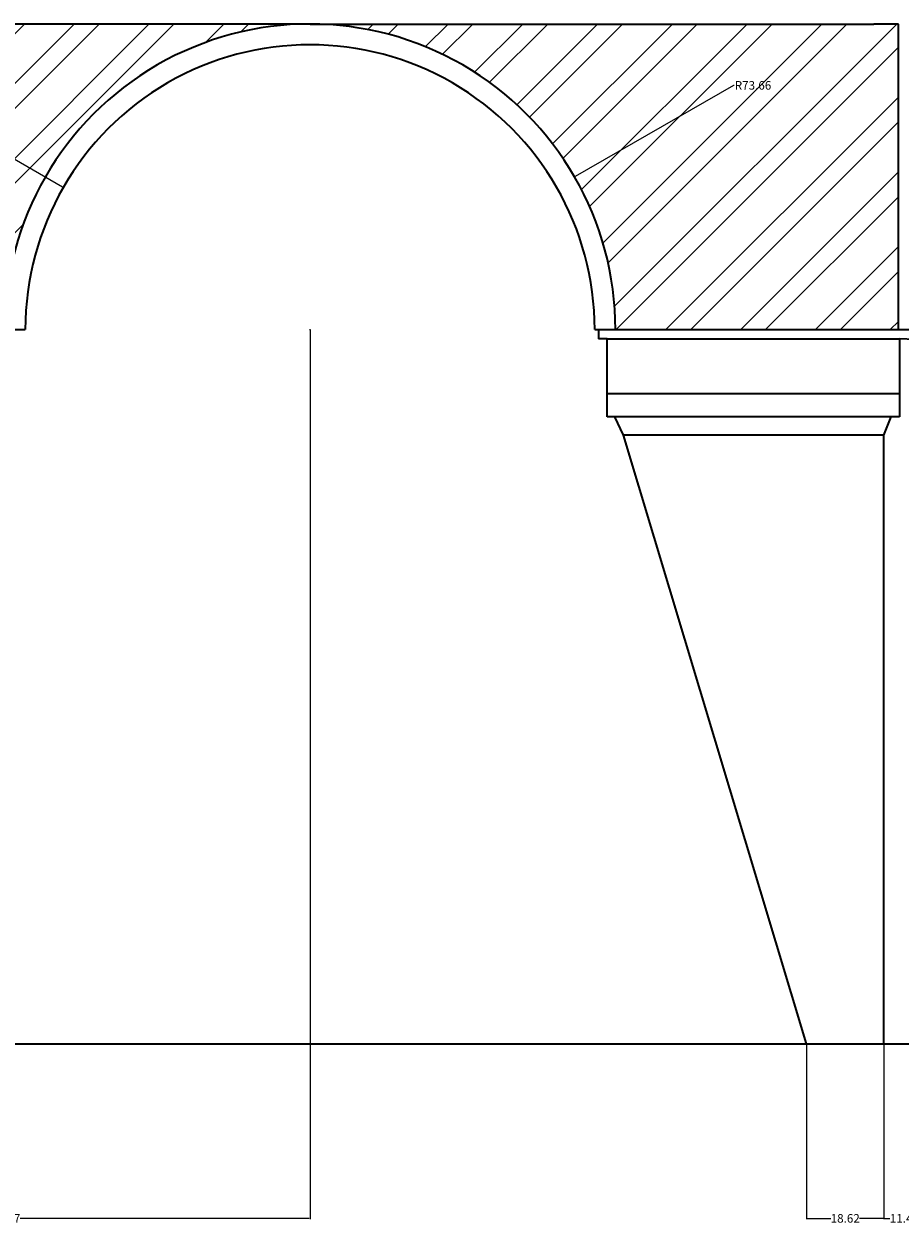
# Model space of a CAD drawing. Units: inches. Extents: x 14 to 859, y 52 to 711.
# Tile 3 of 11: x 366 to 577, y 52 to 342. Entities that reach past the tile are written whole.
import ezdxf

# ---------------------------------------------------------------- set-up
doc = ezdxf.new("R2010")
doc.units = ezdxf.units.IN
doc.header["$MEASUREMENT"] = 0
for name, color, linetype, lineweight in [('A-ANNO-DIMS', 2, 'Continuous', 18), ('A-ELEV', 7, 'Continuous', 35), ('A-ELEV-PATT', 8, 'Continuous', 13)]:
    doc.layers.add(name, color=color, linetype=linetype, lineweight=lineweight)
doc.styles.get("Standard").update_dxf_attribs({"font": 'arial.ttf'})
doc.dimstyles.get("Standard").update_dxf_attribs({"dimtxt": 2.0625, "dimasz": 0.18, "dimexe": 0.18, "dimexo": 0.0625, "dimgap": 0.09, "dimtad": 0, "dimtih": 1, "dimtoh": 1, "dimdec": 4, "dimzin": 0, "dimdsep": 46, "dimlunit": 4, "dimtxsty": 'Standard', "dimcen": 0.09, "dimadec": 0, "dimazin": 0, "dimtfac": 1, "dimtdec": 4, "dimtofl": 0, "dimtmove": 0, "dimatfit": 3, "dimfxl": 1, "dimtolj": 1, "dimtzin": 0, "dimarcsym": 0})

# ---------------------------------------------------------------- blocks, each defined once
blk = doc.blocks.new('*D13')
at = {"layer": 'A-ANNO-DIMS', "color": 0, "lineweight": -2, "transparency": 16777216}
for p, q in [((60.78, 339.73), (60.78, 709.71)), ((60.96, 709.53), (432.6, 709.53)), ((811.37, 709.53), (439.73, 709.53)), ((811.55, 339.73), (811.55, 709.71))]:
    blk.add_line(p, q, dxfattribs=at)
at = {"layer": 'A-ANNO-DIMS', "color": 0, "transparency": 16777216}
for points in [[(60.96, 709.56), (60.96, 709.5), (60.78, 709.53)], [(811.37, 709.56), (811.37, 709.5), (811.55, 709.53)]]:
    blk.add_solid(points, dxfattribs=at)
at = {"layer": 'Defpoints', "color": 0, "transparency": 16777216}
for p in [(811.55, 709.53), (60.78, 339.66), (811.55, 339.66)]:
    blk.add_point(p, dxfattribs=at)
at = {"layer": 'A-ANNO-DIMS', "color": 0, "transparency": 16777216, "insert": (436.17, 709.53), "char_height": 2.062, "attachment_point": 5}
blk.add_mtext('\\A1;750.8', dxfattribs=at)
blk = doc.blocks.new('*D16')
at = {"layer": 'A-ANNO-DIMS', "color": 0, "lineweight": -2, "transparency": 16777216}
for p, q in [((429.96, 670.76), (17.7, 670.76)), ((17.88, 670.58), (17.88, 384.41)), ((17.88, 95.97), (17.88, 382.14)), ((60.72, 95.79), (17.7, 95.79))]:
    blk.add_line(p, q, dxfattribs=at)
at = {"layer": 'A-ANNO-DIMS', "color": 0, "transparency": 16777216}
for points in [[(17.85, 670.58), (17.91, 670.58), (17.88, 670.76)], [(17.85, 95.97), (17.91, 95.97), (17.88, 95.79)]]:
    blk.add_solid(points, dxfattribs=at)
at = {"layer": 'Defpoints', "color": 0, "transparency": 16777216}
for p in [(17.88, 670.76), (430.02, 670.76), (60.78, 95.79)]:
    blk.add_point(p, dxfattribs=at)
at = {"layer": 'A-ANNO-DIMS', "color": 0, "transparency": 16777216, "insert": (17.88, 383.28), "char_height": 2.062, "attachment_point": 5}
blk.add_mtext('\\A1;575', dxfattribs=at)
blk = doc.blocks.new('*D24')
at = {"layer": 'A-ANNO-DIMS', "color": 0, "lineweight": -2, "transparency": 16777216}
for p, q in [((434.6, 267.95), (434.6, 53.56)), ((287.89, 95.73), (287.89, 53.56)), ((288.07, 53.74), (357.77, 53.74)), ((434.42, 53.74), (364.72, 53.74))]:
    blk.add_line(p, q, dxfattribs=at)
at = {"layer": 'A-ANNO-DIMS', "color": 0, "transparency": 16777216}
for points in [[(288.07, 53.77), (288.07, 53.71), (287.89, 53.74)], [(434.42, 53.77), (434.42, 53.71), (434.6, 53.74)]]:
    blk.add_solid(points, dxfattribs=at)
at = {"layer": 'Defpoints', "color": 0, "transparency": 16777216}
for p in [(434.6, 268.01), (287.89, 95.79), (434.6, 53.74)]:
    blk.add_point(p, dxfattribs=at)
at = {"layer": 'A-ANNO-DIMS', "color": 0, "transparency": 16777216, "insert": (361.24, 53.74), "char_height": 2.062, "attachment_point": 5}
blk.add_mtext('\\A1;146.7', dxfattribs=at)
blk = doc.blocks.new('*D33')
at = {"layer": 'A-ANNO-DIMS', "color": 0, "lineweight": -2, "transparency": 16777216}
for p, q in [((554.36, 95.73), (554.36, 53.56)), ((572.98, 95.73), (572.98, 53.56)), ((554.54, 53.74), (560.21, 53.74)), ((572.8, 53.74), (567.13, 53.74))]:
    blk.add_line(p, q, dxfattribs=at)
at = {"layer": 'A-ANNO-DIMS', "color": 0, "transparency": 16777216}
for points in [[(554.54, 53.77), (554.54, 53.71), (554.36, 53.74)], [(572.8, 53.77), (572.8, 53.71), (572.98, 53.74)]]:
    blk.add_solid(points, dxfattribs=at)
at = {"layer": 'Defpoints', "color": 0, "transparency": 16777216}
for p in [(554.36, 95.79), (572.98, 95.79), (572.98, 53.74)]:
    blk.add_point(p, dxfattribs=at)
at = {"layer": 'A-ANNO-DIMS', "color": 0, "transparency": 16777216, "insert": (563.67, 53.74), "char_height": 2.062, "attachment_point": 5}
blk.add_mtext('\\A1;18.62', dxfattribs=at)
blk = doc.blocks.new('*D34')
at = {"layer": 'A-ANNO-DIMS', "color": 0, "lineweight": -2, "transparency": 16777216}
for p, q in [((572.98, 95.73), (572.98, 53.56)), ((584.44, 95.73), (584.44, 53.56)), ((573.16, 53.74), (574.44, 53.74)), ((584.26, 53.74), (582.98, 53.74))]:
    blk.add_line(p, q, dxfattribs=at)
at = {"layer": 'A-ANNO-DIMS', "color": 0, "transparency": 16777216}
for points in [[(573.16, 53.77), (573.16, 53.71), (572.98, 53.74)], [(584.26, 53.77), (584.26, 53.71), (584.44, 53.74)]]:
    blk.add_solid(points, dxfattribs=at)
at = {"layer": 'Defpoints', "color": 0, "transparency": 16777216}
for p in [(572.98, 95.79), (584.44, 95.79), (584.44, 53.74)]:
    blk.add_point(p, dxfattribs=at)
at = {"layer": 'A-ANNO-DIMS', "color": 0, "transparency": 16777216, "insert": (578.71, 53.74), "char_height": 2.062, "attachment_point": 5}
blk.add_mtext('\\A1;11.463', dxfattribs=at)
blk = doc.blocks.new('*D125')
at = {"layer": 'A-ANNO-DIMS', "color": 0, "lineweight": -2, "transparency": 16777216}
for p, q in [((536.7, 326.88), (498.57, 304.9)), ((536.88, 326.88), (536.7, 326.88)), ((434.51, 268.01), (434.69, 268.01)), ((434.6, 267.92), (434.6, 268.1))]:
    blk.add_line(p, q, dxfattribs=at)
at = {"layer": 'A-ANNO-DIMS', "color": 0, "transparency": 16777216}
blk.add_solid([(498.55, 304.92), (498.58, 304.87), (498.41, 304.81)], dxfattribs=at)
at = {"layer": 'Defpoints', "color": 0, "transparency": 16777216}
for p in [(498.41, 304.81), (434.6, 268.01)]:
    blk.add_point(p, dxfattribs=at)
at = {"layer": 'A-ANNO-DIMS', "color": 0, "transparency": 16777216, "insert": (541.43, 326.88), "char_height": 2.062, "attachment_point": 5}
blk.add_mtext('\\A1;R73.66', dxfattribs=at)
blk = doc.blocks.new('*D126')
at = {"layer": 'A-ANNO-DIMS', "color": 0, "lineweight": -2, "transparency": 16777216}
for p, q in [((339.23, 322.87), (339.41, 322.87)), ((339.41, 322.87), (374.95, 302.39)), ((434.51, 268.01), (434.69, 268.01)), ((434.6, 267.92), (434.6, 268.1))]:
    blk.add_line(p, q, dxfattribs=at)
at = {"layer": 'A-ANNO-DIMS', "color": 0, "transparency": 16777216}
blk.add_solid([(374.97, 302.41), (374.94, 302.36), (375.11, 302.3)], dxfattribs=at)
at = {"layer": 'Defpoints', "color": 0, "transparency": 16777216}
for p in [(375.11, 302.3), (434.6, 268.01)]:
    blk.add_point(p, dxfattribs=at)
at = {"layer": 'A-ANNO-DIMS', "color": 0, "transparency": 16777216, "insert": (334.68, 322.87), "char_height": 2.062, "attachment_point": 5}
blk.add_mtext('\\A1;R68.66', dxfattribs=at)

msp = doc.modelspace()

# ---------------------------------------------------------------- hatches: boundary and pattern name
at = {"layer": 'A-ELEV-PATT'}
h = msp.add_hatch(dxfattribs=at)
h.set_pattern_fill('ANSI32', color=256, scale=34)
h.paths.add_polyline_path([(434.5861, 341.6716, 0.41417057), (360.935, 268.0097), (295.7375, 268.0097), (295.7375, 265.9828), (298.7295, 265.9828), (362.2006, 265.9828), (365.3206, 265.8525), (362.2006, 265.8525), (298.7295, 265.9828), (295.7375, 265.9828), (295.7375, 268.0097), (298.7295, 268.0097), (298.7295, 341.6716)])
h.paths.add_polyline_path([(576.5058, 341.6716), (570.5754, 341.6716), (434.5861, 341.6716, -0.41433672), (508.2589, 267.9895), (576.5058, 267.9895)])

# ---------------------------------------------------------------- linework, layer by layer
at = {"layer": 'A-ELEV'}
for p, q in [((434.6078, 341.6716), (298.7295, 341.6716)), ((434.6078, 341.6716), (570.5754, 341.6716)), ((576.5058, 341.6716), (570.5754, 341.6716)), ((576.5058, 267.9895), (576.5058, 341.6716)), ((295.7375, 268.0097), (365.935, 268.0097)), ((503.2589, 267.9895), (580.3801, 267.9895)), ((504.1987, 267.9895), (504.1987, 265.7663)), ((506.2471, 265.7663), (504.1987, 265.7663)), ((506.2471, 252.5803), (506.2471, 265.7663)), ((506.2471, 265.7663), (576.7277, 265.7663)), ((576.7277, 265.7663), (576.7277, 252.5803)), ((580.3801, 265.6361), (576.7277, 265.7663)), ((506.2471, 246.9791), (506.2471, 252.5803)), ((506.2471, 252.5803), (576.7277, 252.5803)), ((576.7277, 252.5803), (576.7277, 246.9791)), ((576.7277, 246.9791), (506.2471, 246.9791)), ((510.1825, 242.5877), (508.0777, 246.9791)), ((572.9779, 242.5877), (574.7583, 246.9791)), ((554.3573, 95.7876), (510.1825, 242.5877)), ((572.9779, 242.5877), (510.1825, 242.5877)), ((572.9779, 95.7876), (572.9779, 242.5877)), ((287.893, 95.7876), (584.4409, 95.7876))]:
    msp.add_line(p, q, dxfattribs=at)
for radius in [73.6619, 68.6619]:
    msp.add_arc((434.5969, 268.0097), radius, 359.983178, 180, dxfattribs=at)

# ---------------------------------------------------------------- dimensions: what is measured, and where the dimension line sits
at = {"layer": 'A-ANNO-DIMS'}
for base, p1, p2, override, picture, middle in [((811.5534, 709.5262), (60.7804, 339.6626), (811.5534, 339.6626), {"dimdec": 1, "dimlfac": 1, "dimrnd": 0, "dimzin": 0, "dimdsep": 46, "dimlunit": 2}, '*D13', (436.1669, 709.5262)), ((434.5969, 53.7364), (287.893, 95.7876), (434.5969, 268.0097), {"dimdec": 1, "dimlfac": 1, "dimrnd": 0, "dimzin": 0, "dimdsep": 46, "dimlunit": 2}, '*D24', (361.245, 53.7364)), ((572.9779, 53.7364), (554.3573, 95.7876), (572.9779, 95.7876), {"dimdec": 2, "dimlfac": 1, "dimrnd": 0, "dimzin": 0, "dimdsep": 46, "dimlunit": 2}, '*D33', (563.6676, 53.7364)), ((584.4409, 53.7364), (572.9779, 95.7876), (584.4409, 95.7876), {"dimdec": 3, "dimlfac": 1, "dimrnd": 0, "dimzin": 0, "dimdsep": 46, "dimlunit": 2}, '*D34', (578.7094, 53.7364))]:
    dim = msp.add_linear_dim(base=base, p1=p1, p2=p2, dimstyle='Standard', override=override, dxfattribs=at)
    dim.commit()
    dim.dimension.update_dxf_attribs({"geometry": picture, "text_midpoint": middle})
dim = msp.add_linear_dim(base=(17.8785, 670.7637), p1=(60.7804, 95.7876), p2=(430.0228, 670.7637), angle=90, dimstyle='Standard', override={"dimdec": 0, "dimlfac": 1, "dimrnd": 0, "dimzin": 0, "dimdsep": 46, "dimlunit": 2}, dxfattribs=at)
dim.commit()
dim.dimension.update_dxf_attribs({"geometry": '*D16', "text_midpoint": (17.8785, 383.2756)})
for mpoint, picture, middle in [((498.4101, 304.8058), '*D125', (541.4342, 326.8835)), ((375.1079, 302.2955), '*D126', (334.6783, 322.8669))]:
    dim = msp.add_radius_dim(center=(434.5969, 268.0097), mpoint=mpoint, dimstyle='Standard', override={"dimdec": 2, "dimlfac": 1, "dimrnd": 0, "dimzin": 0, "dimdsep": 46, "dimlunit": 2}, dxfattribs=at)
    dim.commit()
    dim.dimension.update_dxf_attribs({"geometry": picture, "text_midpoint": middle, "dimtype": 164})

doc.saveas('drawing.dxf')
